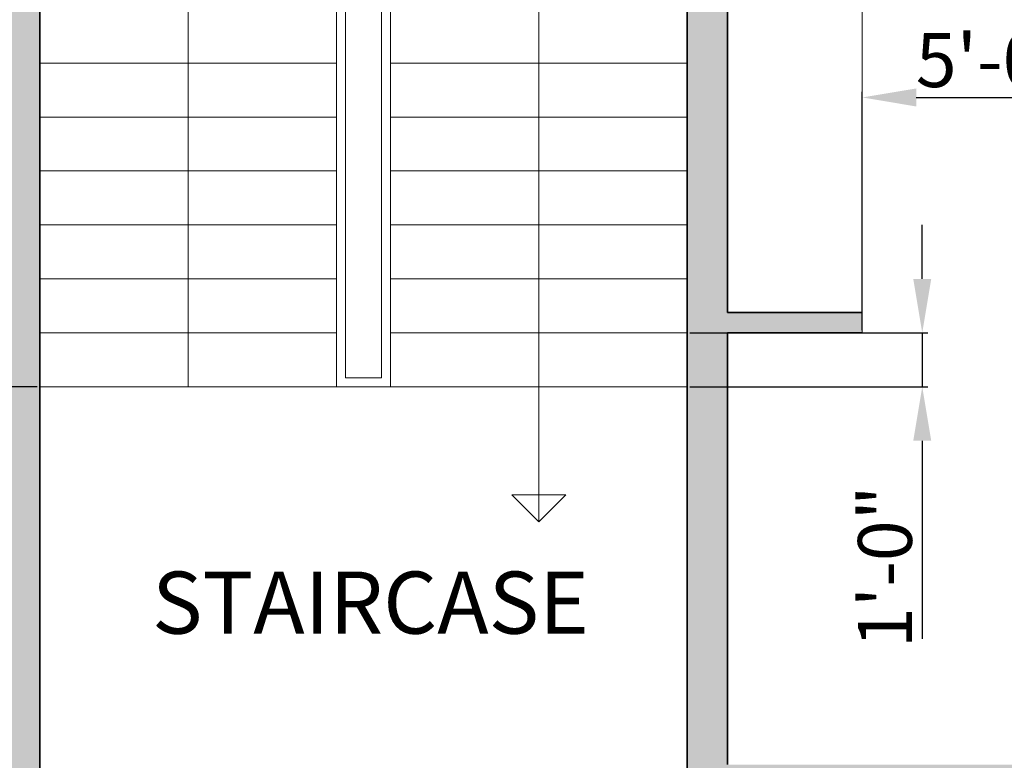
# Model space of a CAD drawing. Units: inches. Extents: x 2083 to 3317, y 1141 to 2115.
# Tile 255 of 256: x 2600 to 2820, y 1713 to 1877. Entities that reach past the tile are written whole.
import ezdxf

# ---------------------------------------------------------------- set-up
doc = ezdxf.new("R2010")
doc.units = ezdxf.units.IN
for name, color, linetype, lineweight in [('A-ANNO-DIMS', 2, 'Continuous', 18), ('A-ANNO-SYMB', 7, 'Continuous', 13), ('A-AREA-IDEN', 7, 'Continuous', 25), ('A-FLOR-CASE', 8, 'Continuous', 18), ('A-FLOR-STRS', 7, 'Continuous', 18), ('A-WALL', 7, 'Continuous', 35)]:
    doc.layers.add(name, color=color, linetype=linetype, lineweight=lineweight)
doc.layers.add('A-WALL-PATT', color=251, linetype='Continuous', lineweight=13, true_color=0x636466)
doc.styles.get("Standard").update_dxf_attribs({"font": 'arial.ttf'})
doc.dimstyles.new('ISO-25', dxfattribs={"dimtxt": 12, "dimasz": 12, "dimexe": 1.25, "dimexo": 0.625, "dimtad": 1, "dimlunit": 3, "dimtxsty": 'Standard', "dimcen": 2.5, "dimadec": 0, "dimazin": 0, "dimtfac": 1, "dimtmove": 0, "dimatfit": 3, "dimfxl": 1, "dimarcsym": 0})

# ---------------------------------------------------------------- blocks, each defined once
blk = doc.blocks.new('*D50')
at = {"layer": 'A-ANNO-DIMS', "color": 0, "lineweight": -2, "transparency": 16777216}
for p, q in [((2604.33, 1939.76), (2551.36, 1939.76)), ((2552.61, 1807.76), (2552.61, 1927.76)), ((2604.33, 1795.76), (2551.36, 1795.76))]:
    blk.add_line(p, q, dxfattribs=at)
at = {"layer": 'A-ANNO-DIMS', "color": 0, "transparency": 16777216}
for points in [[(2550.61, 1927.76), (2554.61, 1927.76), (2552.61, 1939.76)], [(2550.61, 1807.76), (2554.61, 1807.76), (2552.61, 1795.76)]]:
    blk.add_solid(points, dxfattribs=at)
at = {"layer": 'Defpoints', "color": 0, "transparency": 16777216}
for p in [(2552.61, 1939.76), (2604.96, 1939.76), (2604.96, 1795.76)]:
    blk.add_point(p, dxfattribs=at)
at = {"layer": 'A-ANNO-DIMS', "color": 0, "transparency": 16777216, "insert": (2545.86, 1867.76), "char_height": 12, "attachment_point": 5, "rotation": 90}
blk.add_mtext('12\'-0"', dxfattribs=at)
blk = doc.blocks.new('*D52')
at = {"layer": 'A-ANNO-DIMS', "color": 0, "lineweight": -2, "transparency": 16777216}
for p, q in [((2787.96, 1808.39), (2787.96, 1861.36)), ((2847.96, 1808.39), (2847.96, 1861.36)), ((2799.96, 1860.11), (2835.96, 1860.11))]:
    blk.add_line(p, q, dxfattribs=at)
at = {"layer": 'A-ANNO-DIMS', "color": 0, "transparency": 16777216}
for points in [[(2799.96, 1862.11), (2799.96, 1858.11), (2787.96, 1860.11)], [(2835.96, 1862.11), (2835.96, 1858.11), (2847.96, 1860.11)]]:
    blk.add_solid(points, dxfattribs=at)
at = {"layer": 'Defpoints', "color": 0, "transparency": 16777216}
for p in [(2847.96, 1860.11), (2787.96, 1807.76), (2847.96, 1807.76)]:
    blk.add_point(p, dxfattribs=at)
at = {"layer": 'A-ANNO-DIMS', "color": 0, "transparency": 16777216, "insert": (2817.96, 1866.86), "char_height": 12, "attachment_point": 5}
blk.add_mtext('5\'-0"', dxfattribs=at)
blk = doc.blocks.new('*D60')
at = {"layer": 'A-ANNO-DIMS', "color": 0, "lineweight": -2, "transparency": 16777216}
for p, q in [((2801.31, 1819.76), (2801.31, 1831.76)), ((2749.58, 1807.76), (2802.56, 1807.76)), ((2801.31, 1807.76), (2801.31, 1795.76)), ((2749.58, 1795.76), (2802.56, 1795.76)), ((2801.31, 1783.76), (2801.31, 1739.74))]:
    blk.add_line(p, q, dxfattribs=at)
at = {"layer": 'A-ANNO-DIMS', "color": 0, "transparency": 16777216}
for points in [[(2799.31, 1819.76), (2803.31, 1819.76), (2801.31, 1807.76)], [(2799.31, 1783.76), (2803.31, 1783.76), (2801.31, 1795.76)]]:
    blk.add_solid(points, dxfattribs=at)
at = {"layer": 'Defpoints', "color": 0, "transparency": 16777216}
for p in [(2748.96, 1807.76), (2748.96, 1795.76), (2801.31, 1795.76)]:
    blk.add_point(p, dxfattribs=at)
at = {"layer": 'A-ANNO-DIMS', "color": 0, "transparency": 16777216, "insert": (2794.56, 1755.75), "char_height": 12, "attachment_point": 5, "rotation": 90}
blk.add_mtext('1\'-0"', dxfattribs=at)

msp = doc.modelspace()

# ---------------------------------------------------------------- hatches: boundary and pattern name
at = {"layer": 'A-WALL-PATT'}
h = msp.add_hatch(color=256, dxfattribs=at)
h.dxf.hatch_style = 1
h.paths.add_polyline_path([(3126.96, 2020.761), (2748.96, 2020.761), (2604.96, 2020.761), (2226.96, 2020.761), (2226.96, 1702.761), (2466.96, 1702.761), (2466.96, 1582.761), (2418.96, 1582.761), (2418.96, 1477.761), (2226.96, 1477.761), (2226.96, 1263.261), (2544.96, 1263.261), (2544.96, 1411.761), (2604.96, 1411.761), (2685.96, 1411.761), (2685.96, 1420.761), (2604.96, 1420.761), (2604.96, 1573.761), (2604.96, 1702.761), (2604.96, 2011.761), (2748.96, 2011.761), (2748.96, 1702.761), (2862.96, 1702.761), (2862.96, 1621.761), (2871.96, 1621.761), (2871.96, 1702.761), (2883.96, 1702.761), (2883.96, 1706.939, -0.0264593), (2883.96, 1711.761), (2757.96, 1711.761), (2757.96, 1807.761), (2787.96, 1807.761), (2787.96, 1812.261), (2757.96, 1812.261), (2757.96, 2011.761), (2877.96, 2011.761), (2877.96, 1812.261), (2847.96, 1812.261), (2847.96, 1807.761), (2889.836, 1807.761), (2889.836, 1812.261), (2882.46, 1812.261), (2882.46, 2011.761), (3117.96, 2011.761), (3117.96, 1812.261), (2937.836, 1812.261), (2937.836, 1807.761), (2995.71, 1807.761), (2995.71, 1796.118), (3000.21, 1796.118), (3000.21, 1807.761), (3117.96, 1807.761), (3117.96, 1711.761), (3000.21, 1711.761), (3000.21, 1760.118), (2998.573, 1760.118, -0.020711), (2995.71, 1760.118), (2995.71, 1711.761), (2931.96, 1711.761), (2931.96, 1702.761), (3126.96, 1702.761)])
h.paths.add_polyline_path([(2471.46, 2011.761), (2471.46, 1810.011), (2462.717, 1810.011), (2462.717, 1805.511), (2505.96, 1805.511), (2505.96, 1810.011), (2475.96, 1810.011), (2475.96, 2011.761), (2595.96, 2011.761), (2595.96, 1810.011), (2565.96, 1810.011), (2565.96, 1805.511), (2595.96, 1805.511), (2595.96, 1711.761), (2235.96, 1711.761), (2235.96, 1805.511), (2353.71, 1805.511), (2353.71, 1796.054), (2358.21, 1796.054), (2358.21, 1805.511), (2414.717, 1805.511), (2414.717, 1810.011), (2235.96, 1810.011), (2235.96, 2011.761)], flags=16)
h.paths.add_polyline_path([(2270.205, 1994.61), (2270.205, 1970.61), (2246.205, 1970.61), (2246.205, 1994.61)], flags=0)
edge = h.paths.add_edge_path(flags=0)
edge.add_ellipse((2332.027, 1899.798), major_axis=(-3.043, 3.043), ratio=0.1682525, start_angle=-161.33217, end_angle=-156.30711, ccw=False)
edge.add_ellipse((2333.082, 1898.744), major_axis=(-1.055, 1.055), ratio=0.4535321, start_angle=-123.37102, end_angle=-94.15911)
edge = h.paths.add_edge_path(flags=0)
edge.add_ellipse((2332.027, 1968.876), major_axis=(3.043, 3.043), ratio=0.1682525, start_angle=18.66783, end_angle=23.69289)
edge.add_spline(control_points=[(2332.926, 1970.691), (2332.227, 1970.336), (2330.894, 1969.659), (2328.413, 1970.932), (2327.204, 1967.749), (2324.71, 1969.956), (2322.533, 1967.012), (2320.013, 1971.296), (2317.68, 1968.158), (2316.041, 1967.102), (2315.427, 1966.81)], knot_values=[0, 0, 0, 0, 2.2670587, 4.3245589, 6.6855835, 8.8786411, 11.121502, 14.300359, 17.7552837, 19.732645, 19.732645, 19.732645, 19.732645], degree=3, periodic=0)
edge.add_ellipse((2332.027, 1968.876), major_axis=(3.043, 3.043), ratio=0.1682525, start_angle=18.66783, end_angle=23.69289, ccw=False)
edge.add_ellipse((2333.082, 1969.931), major_axis=(1.055, 1.055), ratio=0.4535321, start_angle=56.62898, end_angle=85.84089, ccw=False)
edge = h.paths.add_edge_path(flags=0)
edge.add_spline(control_points=[(2296.428, 1967.988), (2293.628, 1965.336), (2287.704, 1959.727), (2299.744, 1949.996), (2294.533, 1935.669), (2290.573, 1920.604), (2293.394, 1909.974), (2296.185, 1904.967)], knot_values=[0.0991853, 0.0991853, 0.0991853, 0.0991853, 0.3453009, 0.6198217, 0.9826526, 1.3860932, 1.8105546, 1.8105546, 1.8105546, 1.8105546], degree=3, periodic=0)
edge.add_spline(control_points=[(2296.185, 1904.967), (2297.384, 1902.619), (2298.001, 1901.949), (2298.553, 1901.468)], knot_values=[0.0062457, 0.0062457, 0.0062457, 0.0062457, 0.0554759, 0.0554759, 0.0554759, 0.0554759], degree=3, periodic=0)
edge.add_spline(control_points=[(2298.553, 1901.468), (2297.259, 1900.923), (2295.225, 1900.232), (2293.06, 1900.614), (2292.101, 1900.788), (2292.09, 1900.791)], knot_values=[0.3128349, 0.3128349, 0.3128349, 0.3128349, 0.4017797, 0.4749867, 0.4759027, 0.4759027, 0.4759027, 0.4759027], degree=3, periodic=0)
edge.add_arc((2292.794, 1904.664), 3.937, 215.4209, 259.69818, ccw=False)
edge.add_spline(control_points=[(2289.585, 1902.382), (2289.477, 1902.535), (2289.368, 1902.688), (2289.261, 1902.841)], knot_values=[0.1028719, 0.1028719, 0.1028719, 0.1028719, 0.1168958, 0.1168958, 0.1168958, 0.1168958], degree=3, periodic=0)
edge.add_spline(control_points=[(2289.261, 1902.841), (2288.687, 1902.55), (2287.64, 1902.02), (2285.881, 1901.874), (2283.853, 1901.504), (2281.72, 1899.711), (2278.467, 1899.493), (2276.157, 1901.883), (2272.259, 1899.804), (2267.778, 1901.843), (2262.244, 1900.184), (2257.415, 1901.782), (2254.318, 1900.726), (2253.178, 1900.337)], knot_values=[0, 0, 0, 0, 1.9079767, 3.4771759, 5.261074, 7.9728515, 11.6802485, 13.7179214, 16.9395917, 22.789562, 27.5025027, 33.5952153, 37.1456181, 37.1456181, 37.1456181, 37.1456181], degree=3, periodic=0)
edge.add_line((2253.178, 1900.337), (2250.244, 1902.841))
edge.add_line((2250.244, 1902.841), (2250.244, 1965.833))
edge.add_line((2250.244, 1965.833), (2253.178, 1968.337))
edge.add_spline(control_points=[(2253.178, 1968.337), (2254.318, 1967.948), (2257.415, 1966.892), (2262.244, 1968.49), (2267.778, 1966.831), (2271.527, 1968.537), (2273.876, 1967.828), (2274.207, 1967.728)], knot_values=[0, 0, 0, 0, 0.0901802, 0.2449351, 0.3646438, 0.5132331, 0.5378548, 0.5378548, 0.5378548, 0.5378548], degree=3, periodic=0)
edge.add_arc((2274.353, 1963.793), 3.937, 72.05113, 92.12795, ccw=False)
edge.add_arc((2281.297, 1985.23), 18.596, 252.05113, 288.56572)
edge.add_arc((2292.317, 1956.029), 12.646, 71.02679, 113.77822, ccw=False)
edge = h.paths.add_edge_path(flags=0)
edge.add_spline(control_points=[(2274.899, 1951.856), (2275.066, 1951.617), (2275.233, 1951.377), (2275.398, 1951.136)], knot_values=[1.4099157, 1.4099157, 1.4099157, 1.4099157, 1.4315903, 1.4315903, 1.4315903, 1.4315903], degree=3, periodic=0)
edge.add_spline(control_points=[(2275.398, 1951.136), (2275.792, 1950.562), (2276.179, 1949.984), (2276.546, 1949.397)], knot_values=[1.3582378, 1.3582378, 1.3582378, 1.3582378, 1.4099157, 1.4099157, 1.4099157, 1.4099157], degree=3, periodic=0)
edge.add_line((2276.546, 1949.397), (2277.437, 1947.862))
edge.add_spline(control_points=[(2277.437, 1947.862), (2276.304, 1945.673), (2274.64, 1942.427), (2274.632, 1938.094), (2272.799, 1930.852), (2274.356, 1943.897), (2275.948, 1947.923), (2276.546, 1949.397)], knot_values=[0.0056315, 0.0056315, 0.0056315, 0.0056315, 0.1860139, 0.2660015, 0.3570872, 0.5963902, 0.7397317, 0.7397317, 0.7397317, 0.7397317], degree=3, periodic=0)
edge.add_spline(control_points=[(2276.546, 1949.397), (2276.179, 1949.984), (2275.792, 1950.562), (2275.398, 1951.136)], knot_values=[1.3582378, 1.3582378, 1.3582378, 1.3582378, 1.4099157, 1.4099157, 1.4099157, 1.4099157], degree=3, periodic=0)
edge.add_spline(control_points=[(2275.398, 1951.136), (2274.943, 1950.08), (2274.208, 1948.025), (2273.935, 1944.851), (2272.469, 1937.627), (2273.466, 1945.696), (2274.701, 1951.059), (2274.899, 1951.856)], knot_values=[0.1043639, 0.1043639, 0.1043639, 0.1043639, 0.1896363, 0.2696239, 0.3607096, 0.6000126, 0.6446217, 0.6446217, 0.6446217, 0.6446217], degree=3, periodic=0)
h.paths.add_polyline_path([(2269.168, 1963.128, -0.3575267), (2268.171, 1960.976, -0.0925607), (2268.171, 1939.436, -0.3575267), (2269.168, 1937.285, -0.3575267), (2267.016, 1938.282, -0.1647847), (2254.686, 1938.282, -0.3575267), (2252.534, 1937.285, -0.3575267), (2253.531, 1939.436, -0.0925607), (2253.531, 1960.976, -0.3575267), (2252.534, 1963.128, -0.3575267), (2254.686, 1962.131, -0.1647847), (2267.016, 1962.131, -0.3575267)], flags=0)
h.paths.add_polyline_path([(2248.874, 1967.802), (2248.874, 1957.028), (2249.458, 1957.028), (2249.458, 1911.647), (2248.874, 1911.647), (2248.874, 1900.873), (2246.512, 1900.873, 0.1973271), (2244.15, 1902.457), (2244.15, 1966.218, 0.1973271), (2246.512, 1967.802)], flags=0)
h.paths.add_polyline_path([(2269.168, 1931.389, -0.3575267), (2268.171, 1929.238, -0.0925607), (2268.171, 1907.698, -0.3575267), (2269.168, 1905.547, -0.3575267), (2267.016, 1906.544, -0.1647847), (2254.686, 1906.544, -0.3575267), (2252.534, 1905.547, -0.3575267), (2253.531, 1907.698, -0.0925607), (2253.531, 1929.238, -0.3575267), (2252.534, 1931.389, -0.3575267), (2254.686, 1930.392, -0.1647847), (2267.016, 1930.392, -0.3575267)], flags=0)
edge = h.paths.add_edge_path(flags=0)
edge.add_spline(control_points=[(2276.197, 1906.724), (2276.168, 1909.029), (2276.114, 1913.372), (2270.598, 1924.925), (2273.905, 1919.013), (2275.922, 1916.262), (2275.475, 1912.402), (2277.258, 1910.381), (2276.696, 1908.225), (2276.646, 1906.813), (2276.618, 1906.008)], knot_values=[0, 0, 0, 0, 8.6102597, 16.2212739, 18.8430575, 23.8048978, 27.4408283, 29.3561016, 31.2034776, 33.6506866, 33.6506866, 33.6506866, 33.6506866], degree=3, periodic=0)
edge.add_spline(control_points=[(2276.618, 1906.008), (2276.623, 1905.624), (2276.498, 1904.629), (2275.442, 1903.855), (2274.937, 1903.08), (2274.859, 1902.841)], knot_values=[0.1564884, 0.1564884, 0.1564884, 0.1564884, 0.1843975, 0.2313765, 0.2505985, 0.2505985, 0.2505985, 0.2505985], degree=3, periodic=0)
edge.add_line((2274.859, 1902.841), (2276.506, 1902.841))
edge.add_spline(control_points=[(2276.506, 1902.841), (2276.788, 1903.085), (2277.665, 1904.125), (2278.25, 1904.341), (2277.654, 1908.527), (2278.156, 1906.228), (2278.1, 1905.286), (2278.847, 1904.069), (2277.857, 1903.415), (2277.874, 1902.991), (2277.904, 1902.841)], knot_values=[0.0595743, 0.0595743, 0.0595743, 0.0595743, 0.0807529, 0.1037415, 0.1697201, 0.1760361, 0.2071372, 0.2404744, 0.2623409, 0.2736605, 0.2736605, 0.2736605, 0.2736605], degree=3, periodic=0)
edge.add_line((2277.904, 1902.841), (2280.03, 1902.841))
edge.add_spline(control_points=[(2280.03, 1902.841), (2279.888, 1903.088), (2279.499, 1903.982), (2280.152, 1905.939), (2278.104, 1909.658), (2279.762, 1907.185), (2280.328, 1904.875), (2280.485, 1903.49), (2281.463, 1903.249), (2281.758, 1902.936), (2281.834, 1902.841)], knot_values=[0.013856, 0.013856, 0.013856, 0.013856, 0.0348738, 0.0888667, 0.1078792, 0.1267378, 0.158714, 0.1937575, 0.2174868, 0.2267221, 0.2267221, 0.2267221, 0.2267221], degree=3, periodic=0)
edge.add_spline(control_points=[(2281.834, 1902.841), (2281.788, 1902.827), (2281.647, 1902.783), (2281.396, 1902.859), (2281.088, 1902.985), (2280.721, 1903.061), (2280.333, 1903.026), (2280.125, 1902.899), (2280.03, 1902.841)], knot_values=[0, 0, 0, 0, 0.1441304, 0.435517, 0.7492759, 1.1530457, 1.5483707, 1.878348, 1.878348, 1.878348, 1.878348], degree=3, periodic=0)
edge.add_line((2280.03, 1902.841), (2277.904, 1902.841))
edge.add_spline(control_points=[(2277.904, 1902.841), (2277.893, 1902.796), (2277.865, 1902.68), (2277.607, 1902.687), (2277.274, 1902.801), (2276.838, 1902.62), (2276.584, 1902.789), (2276.506, 1902.841)], knot_values=[0, 0, 0, 0, 0.1271885, 0.3261988, 0.6280094, 1.2435704, 1.5153306, 1.5153306, 1.5153306, 1.5153306], degree=3, periodic=0)
edge.add_line((2276.506, 1902.841), (2274.859, 1902.841))
edge.add_spline(control_points=[(2274.859, 1902.841), (2274.814, 1902.899), (2274.725, 1903.013), (2274.493, 1903.119), (2274.244, 1902.961), (2273.937, 1903.185), (2273.614, 1902.983), (2273.408, 1902.883), (2273.322, 1902.841)], knot_values=[0, 0, 0, 0, 0.2184302, 0.4369566, 0.6879766, 0.9903786, 1.3983955, 1.6918498, 1.6918498, 1.6918498, 1.6918498], degree=3, periodic=0)
edge.add_spline(control_points=[(2273.322, 1902.841), (2273.617, 1903.446), (2274.274, 1904.538), (2276.027, 1904.574), (2276.207, 1906.584), (2276.197, 1906.724)], knot_values=[0.0122268, 0.0122268, 0.0122268, 0.0122268, 0.0594721, 0.1062177, 0.134458, 0.134458, 0.134458, 0.134458], degree=3, periodic=0)
h.paths.add_polyline_path([(2270.776, 1897.79), (2270.776, 1873.79), (2246.776, 1873.79), (2246.776, 1897.79)], flags=0)
h.paths.add_polyline_path([(2353.71, 1760.005), (2353.71, 1760.054), (2358.21, 1760.054, -0.033729)], flags=0)
h.paths.add_polyline_path([(2321.819, 1737.529), (2341.995, 1737.529, -0.4142136), (2343.203, 1736.321), (2343.203, 1721.021, -0.4142136), (2341.995, 1719.813), (2321.819, 1719.813, -0.4142136), (2320.611, 1721.021), (2320.611, 1736.321, -0.4142136)], flags=0)
h.paths.add_polyline_path([(2324.235, 1736.321), (2339.579, 1736.321, -0.4142136), (2341.995, 1733.905), (2341.995, 1725.45, -0.4142136), (2339.579, 1723.034), (2333.681, 1723.034), (2333.845, 1722.045, -0.8706461), (2335.425, 1721.826, -0.767327), (2333.923, 1721.423), (2331.291, 1721.423, -0.767327), (2329.788, 1721.826, -0.8706461), (2331.368, 1722.045), (2331.533, 1723.034), (2324.235, 1723.034, -0.4142136), (2321.819, 1725.45), (2321.819, 1733.905, -0.4142136)], flags=0)
h.paths.add_polyline_path([(2570.484, 1928.615), (2589.684, 1928.615), (2590.169, 1928.615), (2590.169, 1904.993), (2570.484, 1904.993)], flags=0)
h.paths.add_polyline_path([(2574.447, 1927.264, -1), (2572.829, 1927.264, -1)], flags=0)
h.paths.add_polyline_path([(2573.09, 1926.941), (2573.925, 1927.776), (2574.148, 1927.553), (2573.313, 1926.718)], flags=0)
h.paths.add_polyline_path([(2578.779, 1919.73, -1), (2571.592, 1919.73, -1)], flags=0)
h.paths.add_polyline_path([(2578.385, 1919.73, -1), (2571.985, 1919.73, -1)], flags=0)
h.paths.add_polyline_path([(2331.596, 1729.476, -1), (2333.618, 1729.476, -1)], flags=0)
h.paths.add_polyline_path([(2578.034, 1927.264, -1), (2576.416, 1927.264, -1)], flags=0)
h.paths.add_polyline_path([(2576.689, 1927.531), (2576.912, 1927.754), (2577.747, 1926.919), (2577.524, 1926.696)], flags=0)
h.paths.add_polyline_path([(2578.139, 1909.86, -1), (2572.232, 1909.86, -1)], flags=0)
h.paths.add_polyline_path([(2577.745, 1909.86, -1), (2572.625, 1909.86, -1)], flags=0)
h.paths.add_polyline_path([(2583.798, 1927.264, -1), (2582.179, 1927.264, -1)], flags=0)
h.paths.add_polyline_path([(2582.719, 1927.754), (2583.554, 1926.919), (2583.331, 1926.696), (2582.496, 1927.531)], flags=0)
h.paths.add_polyline_path([(2582.496, 1927.531), (2582.719, 1927.754), (2583.554, 1926.919), (2583.331, 1926.696)], flags=0)
h.paths.add_polyline_path([(2587.739, 1920.53, -1), (2581.832, 1920.53, -1)], flags=0)
h.paths.add_polyline_path([(2587.345, 1920.53, -1), (2582.225, 1920.53, -1)], flags=0)
h.paths.add_polyline_path([(2587.385, 1927.264, -1), (2585.766, 1927.264, -1)], flags=0)
h.paths.add_polyline_path([(2586.082, 1926.98), (2586.917, 1927.815), (2587.14, 1927.593), (2586.305, 1926.758)], flags=0)
h.paths.add_polyline_path([(2588.379, 1910.66, -1), (2581.192, 1910.66, -1)], flags=0)
h.paths.add_polyline_path([(2587.985, 1910.66, -1), (2581.585, 1910.66, -1)], flags=0)
h.paths.add_polyline_path([(2417.168, 1729.478), (2437.344, 1729.478, -0.4142136), (2438.552, 1728.27), (2438.552, 1712.969, -0.4142136), (2437.344, 1711.761), (2417.168, 1711.761, -0.4142136), (2415.96, 1712.969), (2415.96, 1728.27, -0.4142136)], flags=0)
h.paths.add_polyline_path([(2419.584, 1728.27), (2434.928, 1728.27, -0.4142136), (2437.344, 1725.854), (2437.344, 1717.398, -0.4142136), (2434.928, 1714.983), (2429.029, 1714.983), (2429.194, 1713.994, -0.8706461), (2430.774, 1713.775, -0.767327), (2429.271, 1713.372), (2426.64, 1713.372, -0.767327), (2425.137, 1713.775, -0.8706461), (2426.717, 1713.994), (2426.882, 1714.983), (2419.584, 1714.983, -0.4142136), (2417.168, 1717.398), (2417.168, 1725.854, -0.4142136)], flags=0)
h.paths.add_polyline_path([(2419.584, 1728.27), (2434.928, 1728.27, -0.4142136), (2437.344, 1725.854), (2437.344, 1717.398, -0.4142136), (2434.928, 1714.983), (2429.029, 1714.983), (2428.358, 1719.009), (2427.553, 1719.009), (2426.882, 1714.983), (2419.584, 1714.983, -0.4142136), (2417.168, 1717.398), (2417.168, 1725.854, -0.4142136)], flags=0)
h.paths.add_polyline_path([(2426.944, 1721.425, -1), (2428.967, 1721.425, -1)], flags=0)
h.paths.add_polyline_path([(2475.96, 1702.761), (2595.96, 1702.761), (2595.96, 1582.761), (2475.96, 1582.761)], flags=16)
h.paths.add_polyline_path([(2427.96, 1573.761), (2595.96, 1573.761), (2595.96, 1468.761), (2595.96, 1420.761), (2384.46, 1420.761), (2384.46, 1468.761), (2427.96, 1468.761)], flags=16)
h.paths.add_polyline_path([(2379.96, 1468.761), (2379.96, 1420.761), (2235.96, 1420.761), (2235.96, 1468.761)], flags=16)
h.paths.add_polyline_path([(2317.816, 1466.696), (2337.992, 1466.696, -0.4142136), (2339.2, 1465.488), (2339.2, 1450.187, -0.4142136), (2337.992, 1448.979), (2317.816, 1448.979, -0.4142136), (2316.608, 1450.187), (2316.608, 1465.488, -0.4142136)], flags=0)
h.paths.add_polyline_path([(2320.232, 1465.488), (2335.576, 1465.488, -0.4142136), (2337.992, 1463.072), (2337.992, 1454.616, -0.4142136), (2335.576, 1452.2), (2329.677, 1452.2), (2329.842, 1451.212, -0.8706461), (2331.422, 1450.992, -0.767327), (2329.92, 1450.59), (2327.288, 1450.59, -0.767327), (2325.785, 1450.992, -0.8706461), (2327.365, 1451.212), (2327.53, 1452.2), (2320.232, 1452.2, -0.4142136), (2317.816, 1454.616), (2317.816, 1463.072, -0.4142136)], flags=0)
h.paths.add_polyline_path([(2320.232, 1465.488), (2335.576, 1465.488, -0.4142136), (2337.992, 1463.072), (2337.992, 1454.616, -0.4142136), (2335.576, 1452.2), (2329.677, 1452.2), (2329.006, 1456.227), (2328.201, 1456.227), (2327.53, 1452.2), (2320.232, 1452.2, -0.4142136), (2317.816, 1454.616), (2317.816, 1463.072, -0.4142136)], flags=0)
h.paths.add_polyline_path([(2327.593, 1458.643, -1), (2329.615, 1458.643, -1)], flags=0)
h.paths.add_polyline_path([(2244.412, 1433.34), (2241.921, 1433.34, -0.4142136), (2240.018, 1435.244), (2240.018, 1440.953, -0.4142105), (2241.921, 1442.856), (2244.412, 1442.856, -1.9764724)], flags=0)
h.paths.add_polyline_path([(2245.357, 1434.398, -0.4142136), (2245.357, 1441.799, -2.1440985)], flags=0)
h.paths.add_polyline_path([(2535.96, 1416.261), (2535.96, 1272.261), (2235.96, 1272.261), (2235.96, 1416.261)], flags=16)
h.paths.add_polyline_path([(2260.12, 1384.293), (2260.12, 1362.039), (2237.865, 1362.039), (2237.865, 1384.293)], flags=0)
edge = h.paths.add_edge_path(flags=0)
edge.add_line((2318.252, 1362.093), (2318.146, 1362.001))
edge.add_ellipse((2317.445, 1360.431), major_axis=(2.822, 2.822), ratio=0.1682525, start_angle=18.66783, end_angle=20.94813, ccw=False)
edge.add_ellipse((2318.423, 1361.409), major_axis=(0.978, 0.978), ratio=0.4535321, start_angle=56.62898, end_angle=70.2262, ccw=False)
edge = h.paths.add_edge_path(flags=0)
edge.add_line((2319.107, 1295.571), (2319.015, 1295.677))
edge.add_ellipse((2317.445, 1296.378), major_axis=(-2.822, 2.822), ratio=0.1682525, start_angle=-161.33217, end_angle=-159.05187, ccw=False)
edge.add_ellipse((2318.423, 1295.4), major_axis=(-0.978, 0.978), ratio=0.4535321, start_angle=-123.37102, end_angle=-109.7738)
edge = h.paths.add_edge_path(flags=0)
edge.add_spline(control_points=[(2284.21, 1301.17), (2284.581, 1300.445), (2284.891, 1299.892), (2285.16, 1299.461)], knot_values=[0.0390658, 0.0390658, 0.0390658, 0.0390658, 0.0554759, 0.0554759, 0.0554759, 0.0554759], degree=3, periodic=0)
edge.add_line((2285.16, 1299.461), (2284.21, 1301.17))
edge = h.paths.add_edge_path(flags=0)
edge.add_line((2280.412, 1297.298), (2283.37, 1297.036))
edge.add_line((2283.37, 1297.036), (2286.406, 1297.926))
edge.add_spline(control_points=[(2286.406, 1297.926), (2285.305, 1297.463), (2284.345, 1297.129), (2283.37, 1297.036)], knot_values=[0.3943688, 0.3943688, 0.3943688, 0.3943688, 0.4759027, 0.4759027, 0.4759027, 0.4759027], degree=3, periodic=0)
edge.add_spline(control_points=[(2283.37, 1297.036), (2283.281, 1297.028), (2282.316, 1296.957), (2281.313, 1297.134), (2280.423, 1297.296), (2280.412, 1297.298)], knot_values=[0.3128349, 0.3128349, 0.3128349, 0.3128349, 0.3202458, 0.3934528, 0.3943688, 0.3943688, 0.3943688, 0.3943688], degree=3, periodic=0)
edge = h.paths.add_edge_path(flags=0)
edge.add_line((2284.436, 1359.607), (2280.446, 1355.328))
edge.add_line((2280.446, 1355.328), (2279.58, 1351.018))
edge.add_line((2279.58, 1351.018), (2282.413, 1346.58))
edge.add_spline(control_points=[(2282.413, 1346.58), (2283.153, 1345.589), (2284.253, 1344.029), (2284.801, 1342.387), (2284.935, 1341.806)], knot_values=[1.2400982, 1.2400982, 1.2400982, 1.2400982, 1.3328922, 1.3827123, 1.3827123, 1.3827123, 1.3827123], degree=3, periodic=0)
edge.add_spline(control_points=[(2284.935, 1341.806), (2285.319, 1340.141), (2285.233, 1338.409), (2284.91, 1336.654)], knot_values=[1.0974841, 1.0974841, 1.0974841, 1.0974841, 1.2400982, 1.2400982, 1.2400982, 1.2400982], degree=3, periodic=0)
edge.add_spline(control_points=[(2284.91, 1336.654), (2284.587, 1334.899), (2284.027, 1333.12), (2283.463, 1331.361)], knot_values=[0.9548699, 0.9548699, 0.9548699, 0.9548699, 1.0974841, 1.0974841, 1.0974841, 1.0974841], degree=3, periodic=0)
edge.add_line((2283.463, 1331.361), (2281.89, 1326.153))
edge.add_line((2281.89, 1326.153), (2280.756, 1321.056))
edge.add_line((2280.756, 1321.056), (2280.299, 1316.002))
edge.add_line((2280.299, 1316.002), (2280.716, 1310.95))
edge.add_line((2280.716, 1310.95), (2282.028, 1305.972))
edge.add_line((2282.028, 1305.972), (2284.21, 1301.17))
edge.add_spline(control_points=[(2284.21, 1301.17), (2283.341, 1302.73), (2282.612, 1304.336), (2282.028, 1305.972)], knot_values=[0.0991853, 0.0991853, 0.0991853, 0.0991853, 0.2417994, 0.2417994, 0.2417994, 0.2417994], degree=3, periodic=0)
edge.add_spline(control_points=[(2282.028, 1305.972), (2281.444, 1307.608), (2281.005, 1309.273), (2280.716, 1310.95)], knot_values=[0.2417994, 0.2417994, 0.2417994, 0.2417994, 0.3844135, 0.3844135, 0.3844135, 0.3844135], degree=3, periodic=0)
edge.add_spline(control_points=[(2280.716, 1310.95), (2280.433, 1312.588), (2280.289, 1314.277), (2280.299, 1315.962), (2280.299, 1316.002)], knot_values=[0.3844135, 0.3844135, 0.3844135, 0.3844135, 0.5236467, 0.5270276, 0.5270276, 0.5270276, 0.5270276], degree=3, periodic=0)
edge.add_spline(control_points=[(2280.299, 1316.002), (2280.312, 1317.687), (2280.478, 1319.368), (2280.756, 1321.056)], knot_values=[0.5270276, 0.5270276, 0.5270276, 0.5270276, 0.6696417, 0.6696417, 0.6696417, 0.6696417], degree=3, periodic=0)
edge.add_spline(control_points=[(2280.756, 1321.056), (2281.035, 1322.744), (2281.426, 1324.44), (2281.89, 1326.153)], knot_values=[0.6696417, 0.6696417, 0.6696417, 0.6696417, 0.8122558, 0.8122558, 0.8122558, 0.8122558], degree=3, periodic=0)
edge.add_spline(control_points=[(2281.89, 1326.153), (2282.264, 1327.533), (2282.788, 1329.262), (2283.353, 1331.018), (2283.463, 1331.361)], knot_values=[0.8122558, 0.8122558, 0.8122558, 0.8122558, 0.9270873, 0.9548699, 0.9548699, 0.9548699, 0.9548699], degree=3, periodic=0)
edge.add_line((2283.463, 1331.361), (2284.91, 1336.654))
edge.add_line((2284.91, 1336.654), (2284.935, 1341.806))
edge.add_line((2284.935, 1341.806), (2282.413, 1346.58))
edge.add_spline(control_points=[(2282.413, 1346.58), (2281.275, 1348.104), (2280.078, 1349.57), (2279.58, 1351.018)], knot_values=[1.3827123, 1.3827123, 1.3827123, 1.3827123, 1.5253264, 1.5253264, 1.5253264, 1.5253264], degree=3, periodic=0)
edge.add_spline(control_points=[(2279.58, 1351.018), (2279.443, 1351.415), (2279.136, 1352.857), (2279.735, 1354.29), (2280.446, 1355.328)], knot_values=[1.5253264, 1.5253264, 1.5253264, 1.5253264, 1.564439, 1.6679405, 1.6679405, 1.6679405, 1.6679405], degree=3, periodic=0)
edge.add_spline(control_points=[(2280.446, 1355.328), (2281.426, 1356.758), (2282.931, 1358.183), (2284.436, 1359.607)], knot_values=[1.6679405, 1.6679405, 1.6679405, 1.6679405, 1.8105546, 1.8105546, 1.8105546, 1.8105546], degree=3, periodic=0)
edge.add_arc((2280.623, 1348.518), 11.726, 71.02679, 113.77822)
edge.add_arc((2270.405, 1375.595), 17.244, 252.05113, 288.56572, ccw=False)
edge.add_arc((2263.966, 1355.718), 3.651, 72.05113, 92.12795)
edge.add_arc((2263.966, 1355.718), 3.651, 92.12795, 177.98513)
edge.add_spline(control_points=[(2260.318, 1355.846), (2260.26, 1354.221), (2260.551, 1350.187), (2262.999, 1346.766), (2264.473, 1344.649)], knot_values=[1.4315903, 1.4315903, 1.4315903, 1.4315903, 1.5641438, 1.7706953, 1.7706953, 1.7706953, 1.7706953], degree=3, periodic=0)
edge.add_line((2264.473, 1344.649), (2264.936, 1343.983))
edge.add_spline(control_points=[(2263.801, 1340.248), (2263.843, 1340.514), (2264.067, 1341.756), (2264.513, 1343.002), (2264.935, 1343.981)], knot_values=[0.5365702, 0.5365702, 0.5365702, 0.5365702, 0.5593494, 0.6446217, 0.6446217, 0.6446217, 0.6446217], degree=3, periodic=0)
edge.add_spline(control_points=[(2264.935, 1343.981), (2265.118, 1343.715), (2265.299, 1343.448), (2265.477, 1343.179)], knot_values=[1.3840767, 1.3840767, 1.3840767, 1.3840767, 1.4099157, 1.4099157, 1.4099157, 1.4099157], degree=3, periodic=0)
edge.add_spline(control_points=[(2265.477, 1343.179), (2265.655, 1342.911), (2265.829, 1342.641), (2265.999, 1342.369)], knot_values=[1.3582378, 1.3582378, 1.3582378, 1.3582378, 1.3840767, 1.3840767, 1.3840767, 1.3840767], degree=3, periodic=0)
edge.add_line((2265.999, 1342.369), (2266.826, 1340.946))
edge.add_spline(control_points=[(2266.826, 1340.946), (2268.894, 1337.09), (2271.398, 1325.843), (2270.516, 1310.569), (2275.919, 1301.861), (2277.79, 1299.199)], knot_values=[0.1168958, 0.1168958, 0.1168958, 0.1168958, 0.4729873, 1.0509689, 1.3137934, 1.3137934, 1.3137934, 1.3137934], degree=3, periodic=0)
edge.add_spline(control_points=[(2277.79, 1299.199), (2277.839, 1299.128), (2277.889, 1299.057), (2277.94, 1298.987)], knot_values=[0.1098839, 0.1098839, 0.1098839, 0.1098839, 0.1168958, 0.1168958, 0.1168958, 0.1168958], degree=3, periodic=0)
edge.add_line((2277.94, 1298.987), (2277.789, 1299.199))
edge.add_spline(control_points=[(2277.789, 1299.199), (2277.257, 1298.929), (2276.286, 1298.438), (2275.039, 1298.334), (2274.383, 1298.239), (2274.215, 1298.209)], knot_values=[33.1218702, 33.1218702, 33.1218702, 33.1218702, 35.0290557, 36.5982549, 37.1448269, 37.1448269, 37.1448269, 37.1448269], degree=3, periodic=0)
edge.add_line((2274.215, 1298.209), (2273.073, 1297.893))
edge.add_spline(control_points=[(2273.073, 1297.893), (2272.323, 1297.58), (2271.039, 1296.511), (2269.248, 1296.226), (2268.423, 1296.375)], knot_values=[26.5325843, 26.5325843, 26.5325843, 26.5325843, 29.198919, 31.8391012, 31.8391012, 31.8391012, 31.8391012], degree=3, periodic=0)
edge.add_line((2268.423, 1296.375), (2263.879, 1297.458))
edge.add_spline(control_points=[(2263.879, 1297.458), (2263.556, 1297.359), (2261.86, 1296.839), (2260.239, 1297.282), (2258.933, 1297.516)], knot_values=[15.9195506, 15.9195506, 15.9195506, 15.9195506, 16.9395917, 21.2260675, 21.2260675, 21.2260675, 21.2260675], degree=3, periodic=0)
edge.add_line((2258.933, 1297.516), (2254.055, 1297.329))
edge.add_spline(control_points=[(2254.055, 1297.329), (2253.756, 1297.296), (2252.114, 1297.165), (2250.462, 1297.544), (2249.13, 1297.668)], knot_values=[5.3065169, 5.3065169, 5.3065169, 5.3065169, 6.2764352, 10.6130337, 10.6130337, 10.6130337, 10.6130337], degree=3, periodic=0)
edge.add_line((2249.13, 1297.668), (2244.332, 1296.878))
edge.add_line((2244.332, 1296.878), (2241.611, 1299.199))
edge.add_line((2241.611, 1299.199), (2241.611, 1357.609))
edge.add_line((2241.611, 1357.609), (2244.332, 1359.931))
edge.add_line((2244.332, 1359.931), (2252.729, 1359.543))
edge.add_spline(control_points=[(2252.729, 1359.543), (2252.871, 1359.546), (2253.306, 1359.548), (2253.74, 1359.514), (2254.032, 1359.482)], knot_values=[0.233291, 0.233291, 0.233291, 0.233291, 0.2449351, 0.2689274, 0.2689274, 0.2689274, 0.2689274], degree=3, periodic=0)
edge.add_line((2254.032, 1359.482), (2259.587, 1359.416))
edge.add_spline(control_points=[(2259.587, 1359.416), (2260.677, 1359.629), (2262.073, 1359.897), (2263.524, 1359.459), (2263.83, 1359.366)], knot_values=[0.4225164, 0.4225164, 0.4225164, 0.4225164, 0.5132331, 0.5378548, 0.5378548, 0.5378548, 0.5378548], degree=3, periodic=0)
edge.add_arc((2263.966, 1355.718), 3.651, 72.05113, 92.12795, ccw=False)
edge.add_arc((2270.405, 1375.595), 17.244, 252.05113, 288.56572)
edge.add_arc((2280.623, 1348.518), 11.726, 71.02679, 113.77822, ccw=False)
h.paths.add_polyline_path([(2240.341, 1359.435), (2240.341, 1349.444), (2240.882, 1349.444), (2240.882, 1307.365), (2240.341, 1307.365), (2240.341, 1297.374), (2238.15, 1297.374, 0.1973271), (2235.96, 1298.843), (2235.96, 1357.966, 0.1973271), (2238.15, 1359.435)], flags=0)
h.paths.add_polyline_path([(2259.158, 1355.101, -0.3575267), (2258.233, 1353.106, -0.0925607), (2258.233, 1333.133, -0.3575267), (2259.158, 1331.138, -0.3575267), (2257.163, 1332.062, -0.1647847), (2245.729, 1332.062, -0.3575267), (2243.735, 1331.138, -0.3575267), (2244.659, 1333.133, -0.0925607), (2244.659, 1353.106, -0.3575267), (2243.735, 1355.101, -0.3575267), (2245.729, 1354.176, -0.1647847), (2257.163, 1354.176, -0.3575267)], flags=0)
edge = h.paths.add_edge_path(flags=0)
edge.add_line((2265.999, 1342.369), (2266.826, 1340.946))
edge.add_line((2266.826, 1340.946), (2265.308, 1337.814))
edge.add_line((2265.308, 1337.814), (2264.358, 1334.653))
edge.add_line((2264.358, 1334.653), (2264.262, 1333.8))
edge.add_spline(control_points=[(2264.262, 1333.8), (2264.208, 1333.187), (2264.162, 1332.366), (2264.007, 1331.414), (2263.969, 1331.202)], knot_values=[0.4644442, 0.4644442, 0.4644442, 0.4644442, 0.5166905, 0.5316081, 0.5316081, 0.5316081, 0.5316081], degree=3, periodic=0)
edge.add_spline(control_points=[(2263.969, 1331.202), (2263.775, 1330.119), (2263.424, 1328.791), (2263.257, 1328.531), (2263.234, 1328.515)], knot_values=[0.3726816, 0.3726816, 0.3726816, 0.3726816, 0.4488497, 0.4644442, 0.4644442, 0.4644442, 0.4644442], degree=3, periodic=0)
edge.add_spline(control_points=[(2263.234, 1328.515), (2263.096, 1328.42), (2263.131, 1329.301), (2263.275, 1330.616)], knot_values=[0.2809191, 0.2809191, 0.2809191, 0.2809191, 0.3726816, 0.3726816, 0.3726816, 0.3726816], degree=3, periodic=0)
edge.add_spline(control_points=[(2263.275, 1330.616), (2263.419, 1331.93), (2263.672, 1333.677), (2263.97, 1335.315)], knot_values=[0.1891566, 0.1891566, 0.1891566, 0.1891566, 0.2809191, 0.2809191, 0.2809191, 0.2809191], degree=3, periodic=0)
edge.add_spline(control_points=[(2263.97, 1335.315), (2264.1, 1336.032), (2264.419, 1337.622), (2264.755, 1338.864), (2264.947, 1339.491)], knot_values=[0.097394, 0.097394, 0.097394, 0.097394, 0.1375775, 0.1891566, 0.1891566, 0.1891566, 0.1891566], degree=3, periodic=0)
edge.add_spline(control_points=[(2264.947, 1339.491), (2265.29, 1340.606), (2265.644, 1341.494), (2265.999, 1342.369)], knot_values=[0.0056315, 0.0056315, 0.0056315, 0.0056315, 0.097394, 0.097394, 0.097394, 0.097394], degree=3, periodic=0)
h.paths.add_polyline_path([(2259.158, 1325.671, -0.3575267), (2258.233, 1323.676, -0.0925607), (2258.233, 1303.703, -0.3575267), (2259.158, 1301.708, -0.3575267), (2257.163, 1302.633, -0.1647847), (2245.729, 1302.633, -0.3575267), (2243.735, 1301.708, -0.3575267), (2244.659, 1303.703, -0.0925607), (2244.659, 1323.676, -0.3575267), (2243.735, 1325.671, -0.3575267), (2245.729, 1324.747, -0.1647847), (2257.163, 1324.747, -0.3575267)], flags=0)
edge = h.paths.add_edge_path(flags=0)
edge.add_spline(control_points=[(2261.709, 1317.311), (2261.679, 1317.418), (2261.762, 1317.389), (2262.491, 1316.09), (2262.962, 1315.301)], knot_values=[14.9558607, 14.9558607, 14.9558607, 14.9558607, 16.2212739, 18.6948259, 18.6948259, 18.6948259, 18.6948259], degree=3, periodic=0)
edge.add_spline(control_points=[(2262.962, 1315.301), (2262.99, 1315.254), (2263.702, 1314.067), (2264.349, 1313.127), (2264.73, 1312.164)], knot_values=[18.6948259, 18.6948259, 18.6948259, 18.6948259, 18.8430575, 22.433791, 22.433791, 22.433791, 22.433791], degree=3, periodic=0)
edge.add_spline(control_points=[(2264.73, 1312.164), (2264.876, 1311.796), (2265.177, 1310.77), (2265.143, 1309.559), (2265.248, 1308.824)], knot_values=[22.433791, 22.433791, 22.433791, 22.433791, 23.8048978, 26.1727562, 26.1727562, 26.1727562, 26.1727562], degree=3, periodic=0)
edge.add_line((2265.248, 1308.824), (2265.851, 1307.172))
edge.add_spline(control_points=[(2265.851, 1307.172), (2266.065, 1306.822), (2266.384, 1306.332), (2266.424, 1305.781), (2266.42, 1305.611)], knot_values=[28.0625624, 28.0625624, 28.0625624, 28.0625624, 29.3561016, 29.9117214, 29.9117214, 29.9117214, 29.9117214], degree=3, periodic=0)
edge.add_spline(control_points=[(2266.42, 1305.611), (2266.416, 1305.433), (2266.394, 1305.25), (2266.365, 1305.066)], knot_values=[29.9117214, 29.9117214, 29.9117214, 29.9117214, 30.4978371, 30.4978371, 30.4978371, 30.4978371], degree=3, periodic=0)
edge.add_line((2266.365, 1305.066), (2266.066, 1302.136))
edge.add_spline(control_points=[(2266.066, 1302.136), (2266.071, 1301.78), (2265.998, 1301.2), (2265.663, 1300.759), (2265.509, 1300.586)], knot_values=[0.1564884, 0.1564884, 0.1564884, 0.1564884, 0.1843975, 0.2035434, 0.2035434, 0.2035434, 0.2035434], degree=3, periodic=0)
edge.add_line((2265.509, 1300.586), (2264.435, 1299.199))
edge.add_line((2264.435, 1299.199), (2265.962, 1299.199))
edge.add_line((2265.962, 1299.199), (2267.336, 1301.175))
edge.add_line((2267.336, 1301.175), (2267.312, 1301.986))
edge.add_spline(control_points=[(2267.312, 1301.986), (2267.261, 1302.862), (2267.16, 1303.737), (2267.271, 1303.326)], knot_values=[0.1262286, 0.1262286, 0.1262286, 0.1262286, 0.1666174, 0.1666174, 0.1666174, 0.1666174], degree=3, periodic=0)
edge.add_spline(control_points=[(2267.271, 1303.326), (2267.28, 1303.294), (2267.31, 1303.175), (2267.373, 1302.884), (2267.406, 1302.683), (2267.418, 1302.601)], knot_values=[0.1666174, 0.1666174, 0.1666174, 0.1666174, 0.1697201, 0.1760361, 0.1807647, 0.1807647, 0.1807647, 0.1807647], degree=3, periodic=0)
edge.add_spline(control_points=[(2267.744, 1300.988), (2267.688, 1301.151), (2267.481, 1301.657), (2267.484, 1302.145), (2267.418, 1302.601)], knot_values=[0.1807647, 0.1807647, 0.1807647, 0.1807647, 0.1937665, 0.2201389, 0.2201389, 0.2201389, 0.2201389], degree=3, periodic=0)
edge.add_line((2267.418, 1302.601), (2267.744, 1300.988))
edge.add_spline(control_points=[(2267.744, 1300.988), (2267.832, 1300.732), (2267.932, 1300.31), (2267.555, 1299.975), (2267.429, 1299.829)], knot_values=[0.2201389, 0.2201389, 0.2201389, 0.2201389, 0.2404744, 0.2548903, 0.2548903, 0.2548903, 0.2548903], degree=3, periodic=0)
edge.add_line((2267.429, 1299.829), (2267.258, 1299.199))
edge.add_line((2267.258, 1299.199), (2269.23, 1299.199))
edge.add_spline(control_points=[(2269.23, 1299.199), (2269.099, 1299.429), (2268.843, 1300.016), (2269.012, 1300.916), (2268.947, 1301.661)], knot_values=[0.013856, 0.013856, 0.013856, 0.013856, 0.0348738, 0.0670726, 0.0670726, 0.0670726, 0.0670726], degree=3, periodic=0)
edge.add_line((2268.947, 1301.661), (2268.432, 1303.603))
edge.add_spline(control_points=[(2268.432, 1303.603), (2268.176, 1304.192), (2267.596, 1305.251), (2268.041, 1304.623), (2268.251, 1304.282)], knot_values=[0.0901547, 0.0901547, 0.0901547, 0.0901547, 0.1078792, 0.1202891, 0.1202891, 0.1202891, 0.1202891], degree=3, periodic=0)
edge.add_spline(control_points=[(2268.251, 1304.282), (2268.361, 1304.105), (2269.058, 1302.918), (2269.383, 1301.59), (2269.521, 1300.776), (2269.575, 1300.556)], knot_values=[0.1202891, 0.1202891, 0.1202891, 0.1202891, 0.1267378, 0.158714, 0.1735056, 0.1735056, 0.1735056, 0.1735056], degree=3, periodic=0)
edge.add_line((2269.575, 1300.556), (2270.686, 1299.421))
edge.add_spline(control_points=[(2270.686, 1299.421), (2270.767, 1299.357), (2270.838, 1299.281), (2270.903, 1299.199)], knot_values=[0.2181597, 0.2181597, 0.2181597, 0.2181597, 0.2267221, 0.2267221, 0.2267221, 0.2267221], degree=3, periodic=0)
edge.add_line((2270.937, 1299.193), (2270.903, 1299.199))
edge.add_spline(control_points=[(2270.903, 1299.199), (2270.86, 1299.186), (2270.73, 1299.146), (2270.496, 1299.216), (2270.272, 1299.308), (2270.121, 1299.348), (2270.063, 1299.36)], knot_values=[0.939174, 0.939174, 0.939174, 0.939174, 1.0833044, 1.3746911, 1.6884499, 1.878348, 1.878348, 1.878348, 1.878348], degree=3, periodic=0)
edge.add_line((2270.063, 1299.36), (2269.23, 1299.199))
edge.add_line((2269.23, 1299.199), (2267.258, 1299.199))
edge.add_spline(control_points=[(2267.258, 1299.199), (2267.248, 1299.157), (2267.223, 1299.05), (2266.984, 1299.057), (2266.809, 1299.116), (2266.677, 1299.109), (2266.637, 1299.105)], knot_values=[0.7576653, 0.7576653, 0.7576653, 0.7576653, 0.8848538, 1.0838641, 1.3856747, 1.5153306, 1.5153306, 1.5153306, 1.5153306], degree=3, periodic=0)
edge.add_spline(control_points=[(2266.637, 1299.105), (2266.485, 1299.089), (2266.236, 1299.017), (2266.035, 1299.151), (2265.962, 1299.199)], knot_values=[0, 0, 0, 0, 0.4859051, 0.7576653, 0.7576653, 0.7576653, 0.7576653], degree=3, periodic=0)
edge.add_line((2265.962, 1299.199), (2264.435, 1299.199))
edge.add_line((2264.435, 1299.199), (2263.858, 1299.367))
edge.add_spline(control_points=[(2263.858, 1299.367), (2263.819, 1299.371), (2263.78, 1299.386), (2263.74, 1299.402)], knot_values=[0.8459249, 0.8459249, 0.8459249, 0.8459249, 0.9786272, 0.9786272, 0.9786272, 0.9786272], degree=3, periodic=0)
edge.add_line((2263.722, 1299.396), (2263.01, 1299.199))
edge.add_spline(control_points=[(2263.01, 1299.199), (2263.246, 1299.683), (2263.506, 1300.128), (2263.873, 1300.408)], knot_values=[0.0122268, 0.0122268, 0.0122268, 0.0122268, 0.0529705, 0.0529705, 0.0529705, 0.0529705], degree=3, periodic=0)
edge.add_spline(control_points=[(2263.873, 1300.408), (2263.932, 1300.453), (2264.084, 1300.553), (2264.255, 1300.624), (2264.36, 1300.665)], knot_values=[0.0529705, 0.0529705, 0.0529705, 0.0529705, 0.0594721, 0.0690861, 0.0690861, 0.0690861, 0.0690861], degree=3, periodic=0)
edge.add_line((2264.36, 1300.665), (2265.142, 1301.078))
edge.add_line((2265.142, 1301.078), (2265.676, 1302.8))
edge.add_line((2265.676, 1302.8), (2265.541, 1305.704))
edge.add_line((2265.541, 1305.704), (2264.803, 1309.328))
edge.add_line((2264.803, 1309.328), (2263.041, 1314.092))
edge.add_spline(control_points=[(2263.041, 1314.092), (2262.384, 1315.671), (2261.796, 1316.998), (2261.709, 1317.311)], knot_values=[11.2168955, 11.2168955, 11.2168955, 11.2168955, 14.9558607, 14.9558607, 14.9558607, 14.9558607], degree=3, periodic=0)
h.paths.add_polyline_path([(2871.96, 1416.261), (2895.91, 1416.261), (2895.91, 1420.761), (2871.96, 1420.761), (2871.96, 1501.761), (2862.96, 1501.761), (2862.96, 1420.761), (2805.96, 1420.761), (2805.96, 1411.761), (2862.96, 1411.761), (2862.96, 1263.261), (3126.96, 1263.261), (3126.96, 1411.761), (3126.96, 1486.761), (2943.96, 1486.761), (2943.96, 1477.761), (2967.86, 1477.761), (2967.86, 1420.761), (2943.91, 1420.761), (2943.91, 1416.261), (3117.96, 1416.261), (3117.96, 1420.761), (2972.36, 1420.761), (2972.36, 1477.761), (3117.96, 1477.761), (3117.96, 1420.761), (3117.96, 1272.261), (2871.96, 1272.261)], flags=0)
h.paths.add_polyline_path([(2457.126, 1485.943), (2527.603, 1485.943), (2527.603, 1537.636), (2457.126, 1537.636)], flags=8)
h.paths.add_polyline_path([(2481.005, 1609.982), (2590.766, 1609.982), (2590.766, 1682.003), (2481.005, 1682.003)], flags=8)
h.paths.add_polyline_path([(2483.085, 1729.127), (2553.562, 1729.127), (2553.562, 1780.82), (2483.085, 1780.82)], flags=8)

# ---------------------------------------------------------------- linework, layer by layer
at = {"layer": 'A-ANNO-SYMB'}
for p, q in [((2637.96, 1975.761), (2637.96, 1795.761)), ((2715.96, 1975.761), (2715.96, 1771.761)), ((2715.96, 1771.761), (2709.96, 1771.761)), ((2715.96, 1765.761), (2709.96, 1771.761)), ((2715.96, 1771.761), (2721.96, 1771.761)), ((2715.96, 1771.761), (2715.96, 1765.761)), ((2715.96, 1765.761), (2721.96, 1771.761))]:
    msp.add_line(p, q, dxfattribs=at)
at = {"layer": 'A-FLOR-CASE'}
msp.add_line((2787.96, 2011.761), (2787.96, 1807.761), dxfattribs=at)
at = {"layer": 'A-FLOR-STRS'}
for p, q in [((2670.96, 1939.761), (2670.96, 1795.761)), ((2682.96, 1939.761), (2682.96, 1795.761)), ((2672.96, 1937.761), (2672.96, 1797.761)), ((2680.96, 1937.761), (2680.96, 1797.761)), ((2604.96, 1867.761), (2670.96, 1867.761)), ((2682.96, 1867.761), (2748.96, 1867.761)), ((2604.96, 1855.761), (2670.96, 1855.761)), ((2682.96, 1855.761), (2748.96, 1855.761)), ((2604.96, 1843.761), (2670.96, 1843.761)), ((2682.96, 1843.761), (2748.96, 1843.761)), ((2604.96, 1831.761), (2670.96, 1831.761)), ((2682.96, 1831.761), (2748.96, 1831.761)), ((2604.96, 1819.761), (2670.96, 1819.761)), ((2682.96, 1819.761), (2748.96, 1819.761)), ((2604.96, 1807.761), (2670.96, 1807.761)), ((2682.96, 1807.761), (2748.96, 1807.761)), ((2672.96, 1797.761), (2680.96, 1797.761)), ((2604.96, 1795.761), (2748.96, 1795.761))]:
    msp.add_line(p, q, dxfattribs=at)
at = {"layer": 'A-WALL'}
for p, q in [((2604.96, 2011.761), (2604.96, 1702.761)), ((2748.96, 2011.761), (2748.96, 1702.761)), ((2757.96, 2011.761), (2757.96, 1812.261)), ((2757.96, 1812.261), (2787.96, 1812.261)), ((2757.96, 1807.761), (2787.96, 1807.761)), ((2757.96, 1807.761), (2757.96, 1711.761))]:
    msp.add_line(p, q, dxfattribs=at)

# ---------------------------------------------------------------- texts
at = {"layer": 'A-AREA-IDEN', "insert": (2629.918, 1754.668), "char_height": 13.8054, "attachment_point": 1}
msp.add_mtext_dynamic_manual_height_columns('STAIRCASE', width=250.71568, gutter_width=69.027, heights=[0], dxfattribs=at)

# ---------------------------------------------------------------- dimensions: what is measured, and where the dimension line sits
at = {"layer": 'A-ANNO-DIMS'}
for base, p1, p2, angle, picture, middle in [((2552.61, 1939.761), (2604.96, 1795.761), (2604.96, 1939.761), 90, '*D50', (2545.858, 1867.761)), ((2801.31, 1795.761), (2748.96, 1807.761), (2748.96, 1795.761), 270, '*D60', (2794.558, 1755.752))]:
    dim = msp.add_linear_dim(base=base, p1=p1, p2=p2, angle=angle, dimstyle='ISO-25', override={"dimdec": 1, "dimlfac": 1, "dimrnd": 0, "dimzin": 1, "dimdsep": 46, "dimlunit": 4, "dimfrac": 2}, dxfattribs=at)
    dim.commit()
    dim.dimension.update_dxf_attribs({"geometry": picture, "text_midpoint": middle})
dim = msp.add_linear_dim(base=(2847.96, 1860.111), p1=(2787.96, 1807.761), p2=(2847.96, 1807.761), dimstyle='ISO-25', override={"dimdec": 1, "dimlfac": 1, "dimrnd": 0, "dimzin": 1, "dimdsep": 46, "dimlunit": 4, "dimfrac": 2}, dxfattribs=at)
dim.commit()
dim.dimension.update_dxf_attribs({"geometry": '*D52', "text_midpoint": (2817.96, 1866.863)})

doc.saveas('drawing.dxf')
